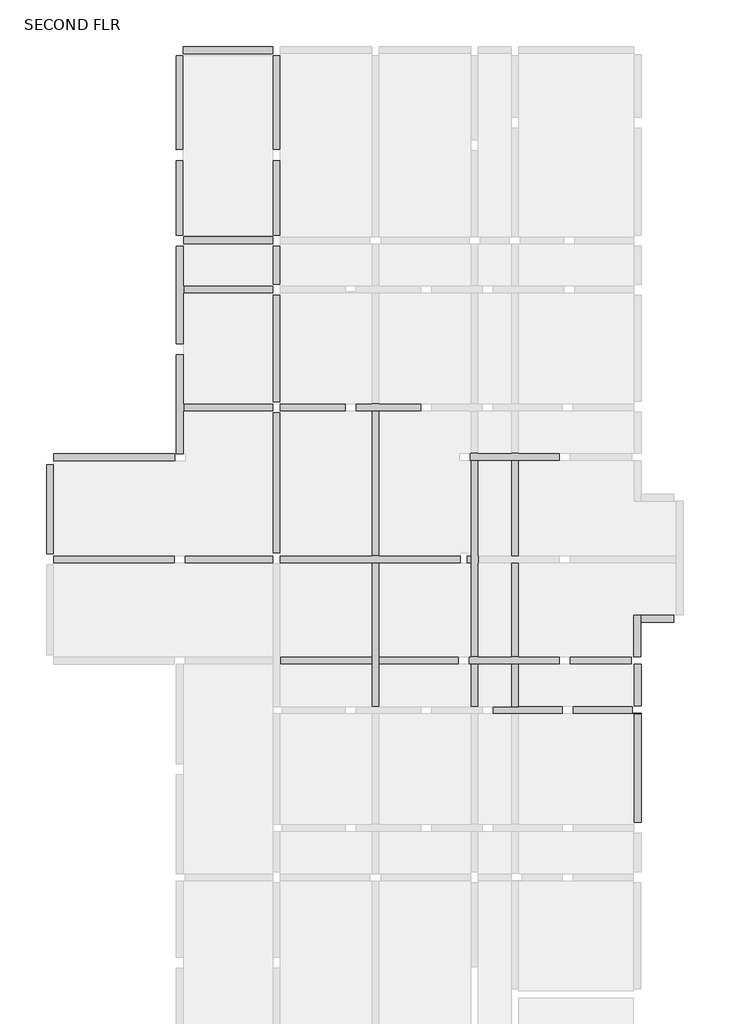
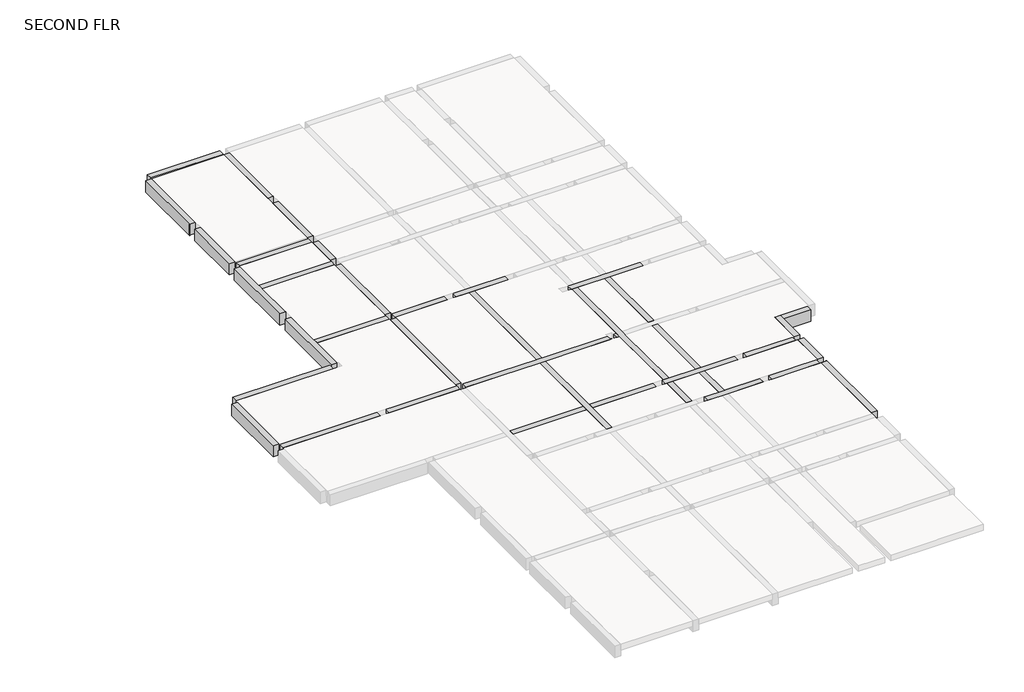
# One storey, part 3 of 4: 39 beams.
"""IFC4 building model written with IfcOpenShell, lengths in millimetres."""

from ifc_helpers import new_model, si_unit, frame, origin, place, context, project, spatial, polyline, outline, extrude, faceted_brep, element, save

model = new_model("IFC4")

# Units and contexts
model_context = context("Model", 3, world=origin())
ifc_project = project(units=[si_unit("LENGTHUNIT", "METRE", prefix="MILLI")], contexts=[model_context])

# Site, building, storey
site = spatial("IfcSite", under=ifc_project)
building = spatial("IfcBuilding", under=site)
storey = spatial("IfcBuildingStorey", under=building, Name="SECOND FLR", Elevation=6048.0)

# Beams
placement = place(None, origin())
element("IfcBeam", 1, ObjectType="M_Concrete-Rectangular Beam : 300 x 600mm", at=placement, inside=storey, context=model_context, shape_type="SweptSolid", body=[
    extrude(outline(polyline([(-1971.7865686, 21837.8349362), (-1971.7865686, 21537.8349362), (-5591.7865686, 21537.8349362), (-5591.7865686, 21837.8349362), (-1971.7865686, 21837.8349362)])), frame((0.0, 0.0, 5448.0), z_axis=(0.0, 0.0, 1.0), x_axis=(1.0, 0.0, 0.0)), (0.0, 0.0, 1.0), 600.0),
])
element("IfcBeam", 2, ObjectType="M_Concrete-Rectangular Beam : 300 x 600mm", at=placement, inside=storey, context=model_context, shape_type="Brep", body=[
    faceted_brep([(-5891.7865686, 21462.8349362, 6048.0), (-5891.7865686, 17662.8349362, 6048.0), (-5888.8105653, 17662.8349362, 6048.0), (-5888.8105653, 17674.7148651, 6048.0), (-5591.7865686, 17674.7148651, 6048.0), (-5591.7865686, 21462.8349362, 6048.0), (-5891.7865686, 21462.8349362, 5448.0), (-5891.7865686, 17662.8349362, 5448.0), (-5591.7865686, 21462.8349362, 5448.0), (-5591.7865686, 17674.7148651, 5448.0), (-5888.8105653, 17674.7148651, 5448.0), (-5888.8105653, 17662.8349362, 5448.0), (-5591.7865686, 17674.7148651, 5748.0), (-5591.7865686, 21462.8349362, 5748.0)], [[[0, 1, 2, 3, 4, 5]], [[1, 0, 6, 7]], [[7, 6, 8, 9, 10, 11]], [[5, 4, 12, 9, 8, 13]], [[8, 6, 0, 5, 13]], [[1, 7, 11, 2]], [[10, 3, 2, 11]], [[3, 10, 9, 12, 4]]]),
])
element("IfcBeam", 3, ObjectType="M_Concrete-Rectangular Beam : 300 x 600mm", at=placement, inside=storey, context=model_context, shape_type="SweptSolid", body=[
    extrude(outline(polyline([(6048.0, -5888.8105653), (5448.0, -5888.8105653), (5448.0, -5588.8105653), (5748.0, -5588.8105653), (5748.0, -5591.7865686), (6048.0, -5591.7865686), (6048.0, -5888.8105653)])), frame((0.0, 14212.5179708, 0.0), z_axis=(0.0, 1.0, 0.0), x_axis=(0.0, 0.0, 1.0)), (0.0, 0.0, 1.0), 3012.1968944),
])
element("IfcBeam", 4, ObjectType="M_Concrete-Rectangular Beam : 300 x 600mm", at=placement, inside=storey, context=model_context, shape_type="Brep", body=[
    faceted_brep([(-5888.8105653, 13762.5179708, 6048.0), (-5888.8105653, 9817.5252033, 6048.0), (-5588.8105653, 9817.5252033, 6048.0), (-5588.8105653, 11857.4075451, 6048.0), (-5588.8105653, 12157.4075451, 6048.0), (-5588.8105653, 13762.5179708, 6048.0), (-5888.8105653, 13762.5179708, 5448.0), (-5888.8105653, 9817.5252033, 5448.0), (-5588.8105653, 13762.5179708, 5448.0), (-5588.8105653, 12157.4075451, 5448.0), (-5588.8105653, 11857.4075451, 5448.0), (-5588.8105653, 9817.5252033, 5448.0), (-5588.8105653, 13762.5179708, 5748.0), (-5588.8105653, 9817.5252033, 5748.0)], [[[0, 1, 2, 3, 4, 5]], [[1, 0, 6, 7]], [[7, 6, 8, 9, 10, 11]], [[11, 10, 9, 8, 12, 5, 4, 3, 2, 13]], [[8, 6, 0, 5, 12]], [[2, 1, 7, 11, 13]]]),
])
element("IfcBeam", 5, ObjectType="M_Concrete-Rectangular Beam : 300 x 600mm", at=placement, inside=storey, context=model_context, shape_type="Brep", body=[
    faceted_brep([(-5888.8105653, 9367.5252033, 6048.0), (-5888.8105653, 5367.5252033, 6048.0), (-5588.8105653, 5367.5252033, 6048.0), (-5588.8105653, 7099.7076276, 6048.0), (-5588.8105653, 7399.7076276, 6048.0), (-5588.8105653, 9367.5252033, 6048.0), (-5888.8105653, 9367.5252033, 5448.0), (-5888.8105653, 5367.5252033, 5448.0), (-5588.8105653, 9367.5252033, 5448.0), (-5588.8105653, 7399.7076276, 5448.0), (-5588.8105653, 7099.7076276, 5448.0), (-5588.8105653, 5367.5252033, 5448.0), (-5588.8105653, 9367.5252033, 5748.0), (-5588.8105653, 5367.5252033, 5748.0)], [[[0, 1, 2, 3, 4, 5]], [[1, 0, 6, 7]], [[7, 6, 8, 9, 10, 11]], [[11, 10, 9, 8, 12, 5, 4, 3, 2, 13]], [[8, 6, 0, 5, 12]], [[2, 1, 7, 11, 13]]]),
])
element("IfcBeam", 6, ObjectType="M_Concrete-Rectangular Beam : 300 x 600mm", at=placement, inside=storey, context=model_context, shape_type="Brep", body=[
    faceted_brep([(-5943.8105653, 5067.6057249, 6048.0), (-5943.8105653, 5367.6057249, 6048.0), (-10828.8105653, 5367.6057249, 6048.0), (-10828.8105653, 5067.6057249, 6048.0), (-5943.8105653, 5367.6057249, 5448.0), (-10828.8105653, 5367.6057249, 5448.0), (-5943.8105653, 5067.6057249, 5448.0), (-10828.8105653, 5067.6057249, 5448.0), (-10828.8105653, 5067.6057249, 5748.0), (-5943.8105653, 5067.6057249, 5748.0)], [[[0, 1, 2, 3]], [[1, 4, 5, 2]], [[4, 6, 7, 5]], [[0, 3, 8, 7, 6, 9]], [[6, 4, 1, 0, 9]], [[3, 2, 5, 7, 8]]]),
])
element("IfcBeam", 7, ObjectType="M_Concrete-Rectangular Beam : 300 x 600mm", at=placement, inside=storey, context=model_context, shape_type="SweptSolid", body=[
    extrude(outline(polyline([(-10828.8105653, 1326.1713929), (-11128.8105653, 1326.1713929), (-11128.8105653, 4932.6057249), (-10828.8105653, 4932.6057249), (-10828.8105653, 1326.1713929)])), frame((0.0, 0.0, 5448.0), z_axis=(0.0, 0.0, 1.0), x_axis=(1.0, 0.0, 0.0)), (0.0, 0.0, 1.0), 600.0),
])
element("IfcBeam", 8, ObjectType="M_Concrete-Rectangular Beam : 300 x 600mm", at=placement, inside=storey, context=model_context, shape_type="Brep", body=[
    faceted_brep([(12619.1163908, -5144.3229916, 6048.0), (12919.1163908, -5144.3229916, 6048.0), (12919.1163908, -5144.3229916, 5448.0), (12619.1163908, -5144.3229916, 5448.0), (12619.1163908, -5151.6229916, 6048.0), (12619.1163908, -9532.1078267, 6048.0), (12919.1163908, -9532.1078267, 6048.0), (12919.1163908, -9532.1078267, 5448.0), (12619.1163908, -9532.1078267, 5448.0), (12619.1163908, -5151.6229916, 5448.0), (12619.1163908, -9532.1078267, 5748.0)], [[[0, 1, 2, 3]], [[1, 0, 4, 5, 6]], [[2, 1, 6, 7]], [[3, 2, 7, 8, 9]], [[0, 3, 9, 8, 10, 5, 4]], [[8, 7, 6, 5, 10]]]),
])
element("IfcBeam", 9, ObjectType="M_Concrete-Rectangular Beam : 300 x 600mm", at=placement, inside=storey, context=model_context, shape_type="Brep", body=[
    faceted_brep([(12619.1163908, -4818.9229916, 5448.0), (12919.1163908, -4818.9229916, 5448.0), (12919.1163908, -4818.9229916, 6048.0), (12619.1163908, -4818.9229916, 6048.0), (12619.1163908, -4818.9229916, 5748.0), (12919.1163908, -3139.4535766, 6048.0), (12619.1163908, -3139.4535766, 6048.0), (12919.1163908, -3139.4535766, 5448.0), (12619.1163908, -3139.4535766, 5448.0), (12619.1163908, -3139.4535766, 5748.0)], [[[0, 1, 2, 3, 4]], [[3, 2, 5, 6]], [[2, 1, 7, 5]], [[1, 0, 8, 7]], [[3, 6, 9, 8, 0, 4]], [[6, 5, 7, 8, 9]]]),
])
element("IfcBeam", 10, ObjectType="M_Concrete-Rectangular Beam : 300 x 600mm", at=placement, inside=storey, context=model_context, shape_type="Brep", body=[
    faceted_brep([(12599.1163908, -2839.4535766, 6048.0), (12899.1163908, -2839.4535766, 6048.0), (12899.1163908, -1448.8286071, 6048.0), (12899.1163908, -1148.8286071, 6048.0), (12599.1163908, -1148.8286071, 6048.0), (12899.1163908, -2839.4535766, 5448.0), (12899.1163908, -1448.8286071, 5448.0), (12899.1163908, -1148.8286071, 5448.0), (12899.1163908, -1148.8286071, 5748.0), (12599.1163908, -2839.4535766, 5448.0), (12599.1163908, -1148.8286071, 5448.0), (12599.1163908, -1148.8286071, 5748.0), (12599.1163908, -2839.4535766, 5748.0)], [[[0, 1, 2, 3, 4]], [[1, 5, 6, 7, 8, 3, 2]], [[5, 9, 10, 7, 6]], [[0, 4, 11, 10, 9, 12]], [[9, 5, 1, 0, 12]], [[4, 3, 8, 7, 10, 11]]]),
])
element("IfcBeam", 11, ObjectType="M_Concrete-Rectangular Beam : 300 x 600mm", at=placement, inside=storey, context=model_context, shape_type="Brep", body=[
    faceted_brep([(14244.1163908, -1448.8286071, 6048.0), (14244.1163908, -1148.8286071, 6048.0), (12899.1163908, -1148.8286071, 6048.0), (12899.1163908, -1448.8286071, 6048.0), (14244.1163908, -1148.8286071, 5748.0), (14244.1163908, -1148.8286071, 5448.0), (12899.1163908, -1148.8286071, 5448.0), (12899.1163908, -1148.8286071, 5748.0), (14244.1163908, -1448.8286071, 5448.0), (12899.1163908, -1448.8286071, 5448.0)], [[[0, 1, 2, 3]], [[2, 1, 4, 5, 6, 7]], [[5, 8, 9, 6]], [[8, 0, 3, 9]], [[0, 8, 5, 4, 1]], [[3, 2, 7, 6, 9]]]),
])
element("IfcBeam", 12, ObjectType="M_Concrete-Rectangular Beam : 300 x 600mm", at=placement, inside=storey, context=model_context, shape_type="Brep", body=[
    faceted_brep([(-1671.7865686, 21462.8349362, 6048.0), (-1971.7865686, 21462.8349362, 6048.0), (-1971.7865686, 17674.7148651, 6048.0), (-1671.7865686, 17674.7148651, 6048.0), (-1971.7865686, 21462.8349362, 5748.0), (-1971.7865686, 21462.8349362, 5448.0), (-1971.7865686, 17674.7148651, 5448.0), (-1971.7865686, 17674.7148651, 5748.0), (-1671.7865686, 21462.8349362, 5448.0), (-1671.7865686, 17674.7148651, 5448.0), (-1671.7865686, 17674.7148651, 5748.0), (-1671.7865686, 21462.8349362, 5748.0)], [[[0, 1, 2, 3]], [[2, 1, 4, 5, 6, 7]], [[5, 8, 9, 6]], [[0, 3, 10, 9, 8, 11]], [[1, 0, 11, 8, 5, 4]], [[3, 2, 7, 6, 9, 10]]]),
])
element("IfcBeam", 13, ObjectType="M_Concrete-Rectangular Beam : 300 x 600mm", at=placement, inside=storey, context=model_context, shape_type="Brep", body=[
    faceted_brep([(-1671.7865686, 17224.7148651, 6048.0), (-1971.7865686, 17224.7148651, 6048.0), (-1971.7865686, 14212.5179708, 6048.0), (-1671.7865686, 14212.5179708, 6048.0), (-1971.7865686, 17224.7148651, 5748.0), (-1971.7865686, 17224.7148651, 5448.0), (-1971.7865686, 14212.5179708, 5448.0), (-1971.7865686, 14212.5179708, 5748.0), (-1671.7865686, 17224.7148651, 5448.0), (-1671.7865686, 14212.5179708, 5448.0), (-1671.7865686, 14212.5179708, 5748.0), (-1671.7865686, 17224.7148651, 5748.0)], [[[0, 1, 2, 3]], [[2, 1, 4, 5, 6, 7]], [[5, 8, 9, 6]], [[0, 3, 10, 9, 8, 11]], [[1, 0, 11, 8, 5, 4]], [[3, 2, 7, 6, 9, 10]]]),
])
element("IfcBeam", 14, ObjectType="M_Concrete-Rectangular Beam : 300 x 600mm", at=placement, inside=storey, context=model_context, shape_type="Brep", body=[
    faceted_brep([(-1671.7865686, 13762.5179708, 6048.0), (-1971.7865686, 13762.5179708, 6048.0), (-1971.7865686, 12232.4075451, 6048.0), (-1671.7865686, 12232.4075451, 6048.0), (-1971.7865686, 13762.5179708, 5748.0), (-1971.7865686, 13762.5179708, 5448.0), (-1971.7865686, 12232.4075451, 5448.0), (-1971.7865686, 12232.4075451, 5748.0), (-1671.7865686, 13762.5179708, 5448.0), (-1671.7865686, 12232.4075451, 5448.0), (-1671.7865686, 12232.4075451, 5748.0), (-1671.7865686, 13762.5179708, 5748.0)], [[[0, 1, 2, 3]], [[2, 1, 4, 5, 6, 7]], [[5, 8, 9, 6]], [[0, 3, 10, 9, 8, 11]], [[1, 0, 11, 8, 5, 4]], [[3, 2, 7, 6, 9, 10]]]),
])
element("IfcBeam", 15, ObjectType="M_Concrete-Rectangular Beam : 300 x 600mm", at=placement, inside=storey, context=model_context, shape_type="Brep", body=[
    faceted_brep([(-1671.7865686, 11782.4075451, 6048.0), (-1971.7865686, 11782.4075451, 6048.0), (-1971.7865686, 7474.7076276, 6048.0), (-1671.7865686, 7474.7076276, 6048.0), (-1971.7865686, 11782.4075451, 5748.0), (-1971.7865686, 11782.4075451, 5448.0), (-1971.7865686, 7474.7076276, 5448.0), (-1971.7865686, 7474.7076276, 5748.0), (-1671.7865686, 11782.4075451, 5448.0), (-1671.7865686, 7474.7076276, 5448.0), (-1671.7865686, 7474.7076276, 5748.0), (-1671.7865686, 11782.4075451, 5748.0)], [[[0, 1, 2, 3]], [[2, 1, 4, 5, 6, 7]], [[5, 8, 9, 6]], [[0, 3, 10, 9, 8, 11]], [[1, 0, 11, 8, 5, 4]], [[3, 2, 7, 6, 9, 10]]]),
])
element("IfcBeam", 16, ObjectType="M_Concrete-Rectangular Beam : 300 x 600mm", at=placement, inside=storey, context=model_context, shape_type="Brep", body=[
    faceted_brep([(-1671.7865686, 7024.7076276, 6048.0), (-1971.7865686, 7024.7076276, 6048.0), (-1971.7865686, 1366.1713929, 6048.0), (-1671.7865686, 1366.1713929, 6048.0), (-1971.7865686, 7024.7076276, 5748.0), (-1971.7865686, 7024.7076276, 5448.0), (-1971.7865686, 1366.1713929, 5448.0), (-1971.7865686, 1366.1713929, 5748.0), (-1671.7865686, 7024.7076276, 5448.0), (-1671.7865686, 1366.1713929, 5448.0), (-1671.7865686, 1366.1713929, 5748.0), (-1671.7865686, 7024.7076276, 5748.0)], [[[0, 1, 2, 3]], [[2, 1, 4, 5, 6, 7]], [[5, 8, 9, 6]], [[0, 3, 10, 9, 8, 11]], [[1, 0, 11, 8, 5, 4]], [[3, 2, 7, 6, 9, 10]]]),
])
element("IfcBeam", 17, ObjectType="M_Concrete-Rectangular Beam : 300 x 600mm", at=placement, inside=storey, context=model_context, shape_type="Brep", body=[
    faceted_brep([(-5588.8105653, 14137.5179708, 6048.0), (-5588.8105653, 13837.5179708, 6048.0), (-1971.7865686, 13837.5179708, 6048.0), (-1971.7865686, 14137.5179708, 6048.0), (-5588.8105653, 13837.5179708, 5748.0), (-5588.8105653, 13837.5179708, 5448.0), (-1971.7865686, 13837.5179708, 5448.0), (-1971.7865686, 13837.5179708, 5748.0), (-5588.8105653, 14137.5179708, 5448.0), (-1971.7865686, 14137.5179708, 5448.0)], [[[0, 1, 2, 3]], [[2, 1, 4, 5, 6, 7]], [[5, 8, 9, 6]], [[8, 0, 3, 9]], [[1, 0, 8, 5, 4]], [[9, 3, 2, 7, 6]]]),
])
element("IfcBeam", 18, ObjectType="M_Concrete-Rectangular Beam : 300 x 600mm", at=placement, inside=storey, context=model_context, shape_type="Brep", body=[
    faceted_brep([(-1971.7865686, 11857.4075451, 6048.0), (-1971.7865686, 12157.4075451, 6048.0), (-5588.8105653, 12157.4075451, 6048.0), (-5588.8105653, 11857.4075451, 6048.0), (-5588.8105653, 11857.4075451, 5748.0), (-5588.8105653, 11857.4075451, 5448.0), (-1971.7865686, 11857.4075451, 5448.0), (-1971.7865686, 11857.4075451, 5748.0), (-1971.7865686, 12157.4075451, 5448.0), (-5588.8105653, 12157.4075451, 5448.0), (-1971.7865686, 12157.4075451, 5748.0), (-5588.8105653, 12157.4075451, 5748.0)], [[[0, 1, 2, 3]], [[0, 3, 4, 5, 6, 7]], [[8, 6, 5, 9]], [[2, 1, 10, 8, 9, 11]], [[1, 0, 7, 6, 8, 10]], [[3, 2, 11, 9, 5, 4]]]),
])
element("IfcBeam", 19, ObjectType="M_Concrete-Rectangular Beam : 300 x 600mm", at=placement, inside=storey, context=model_context, shape_type="Brep", body=[
    faceted_brep([(-1971.7865686, 7099.7076276, 6048.0), (-1971.7865686, 7399.7076276, 6048.0), (-5588.8105653, 7399.7076276, 6048.0), (-5588.8105653, 7099.7076276, 6048.0), (-5588.8105653, 7099.7076276, 5748.0), (-5588.8105653, 7099.7076276, 5448.0), (-1971.7865686, 7099.7076276, 5448.0), (-1971.7865686, 7099.7076276, 5748.0), (-1971.7865686, 7399.7076276, 5448.0), (-5588.8105653, 7399.7076276, 5448.0), (-1971.7865686, 7399.7076276, 5748.0), (-5588.8105653, 7399.7076276, 5748.0)], [[[0, 1, 2, 3]], [[0, 3, 4, 5, 6, 7]], [[8, 6, 5, 9]], [[2, 1, 10, 8, 9, 11]], [[1, 0, 7, 6, 8, 10]], [[3, 2, 11, 9, 5, 4]]]),
])
element("IfcBeam", 20, ObjectType="M_Concrete-Rectangular Beam : 300 x 600mm", at=placement, inside=storey, context=model_context, shape_type="Brep", body=[
    faceted_brep([(-1671.7865686, 7399.7076276, 6048.0), (-1671.7865686, 7099.7076276, 6048.0), (949.7296816, 7099.7076276, 6048.0), (949.7296816, 7399.7076276, 6048.0), (-1671.7865686, 7099.7076276, 5748.0), (-1671.7865686, 7099.7076276, 5448.0), (949.7296816, 7099.7076276, 5448.0), (949.7296816, 7099.7076276, 5748.0), (-1671.7865686, 7399.7076276, 5448.0), (949.7296816, 7399.7076276, 5448.0), (949.7296816, 7399.7076276, 5748.0), (-1671.7865686, 7399.7076276, 5748.0)], [[[0, 1, 2, 3]], [[2, 1, 4, 5, 6, 7]], [[5, 8, 9, 6]], [[0, 3, 10, 9, 8, 11]], [[1, 0, 11, 8, 5, 4]], [[3, 2, 7, 6, 9, 10]]]),
])
element("IfcBeam", 21, ObjectType="M_Concrete-Rectangular Beam : 300 x 600mm", at=placement, inside=storey, context=model_context, shape_type="Brep", body=[
    faceted_brep([(1399.7296816, 7399.7076276, 6048.0), (1399.7296816, 7099.7076276, 6048.0), (2024.7296816, 7099.7076276, 6048.0), (2324.7296816, 7099.7076276, 6048.0), (3997.5248054, 7099.7076276, 6048.0), (3997.5248054, 7399.7076276, 6048.0), (2324.7296816, 7399.7076276, 6048.0), (2024.7296816, 7399.7076276, 6048.0), (1399.7296816, 7099.7076276, 5448.0), (2024.7296816, 7099.7076276, 5448.0), (2324.7296816, 7099.7076276, 5448.0), (3997.5248054, 7099.7076276, 5448.0), (3997.5248054, 7099.7076276, 5748.0), (1399.7296816, 7099.7076276, 5748.0), (1399.7296816, 7399.7076276, 5448.0), (2024.7296816, 7399.7076276, 5448.0), (2324.7296816, 7399.7076276, 5448.0), (3997.5248054, 7399.7076276, 5448.0), (1399.7296816, 7399.7076276, 5748.0), (3997.5248054, 7399.7076276, 5748.0)], [[[0, 1, 2, 3, 4, 5, 6, 7]], [[8, 9, 10, 11, 12, 4, 3, 2, 1, 13]], [[8, 14, 15, 16, 17, 11, 10, 9]], [[17, 16, 15, 14, 18, 0, 7, 6, 5, 19]], [[1, 0, 18, 14, 8, 13]], [[5, 4, 12, 11, 17, 19]]]),
])
element("IfcBeam", 22, ObjectType="M_Concrete-Rectangular Beam : 300 x 600mm", at=placement, inside=storey, context=model_context, shape_type="Brep", body=[
    faceted_brep([(6007.5248054, 5387.6057249, 6048.0), (6007.5248054, 5087.6057249, 6048.0), (6032.5248054, 5087.6057249, 6048.0), (6332.5248054, 5087.6057249, 6048.0), (7656.8679014, 5087.6057249, 6048.0), (7956.8679014, 5087.6057249, 6048.0), (9601.8679014, 5087.6057249, 6048.0), (9601.8679014, 5387.6057249, 6048.0), (7956.8679014, 5387.6057249, 6048.0), (7656.8679014, 5387.6057249, 6048.0), (6332.5248054, 5387.6057249, 6048.0), (6032.5248054, 5387.6057249, 6048.0), (6007.5248054, 5087.6057249, 5448.0), (6032.5248054, 5087.6057249, 5448.0), (6332.5248054, 5087.6057249, 5448.0), (7656.8679014, 5087.6057249, 5448.0), (7956.8679014, 5087.6057249, 5448.0), (9601.8679014, 5087.6057249, 5448.0), (9601.8679014, 5087.6057249, 5748.0), (6007.5248054, 5087.6057249, 5748.0), (6007.5248054, 5387.6057249, 5448.0), (6032.5248054, 5387.6057249, 5448.0), (6332.5248054, 5387.6057249, 5448.0), (7656.8679014, 5387.6057249, 5448.0), (7956.8679014, 5387.6057249, 5448.0), (9601.8679014, 5387.6057249, 5448.0), (6007.5248054, 5387.6057249, 5748.0), (9601.8679014, 5387.6057249, 5748.0)], [[[0, 1, 2, 3, 4, 5, 6, 7, 8, 9, 10, 11]], [[12, 13, 14, 15, 16, 17, 18, 6, 5, 4, 3, 2, 1, 19]], [[12, 20, 21, 22, 23, 24, 25, 17, 16, 15, 14, 13]], [[25, 24, 23, 22, 21, 20, 26, 0, 11, 10, 9, 8, 7, 27]], [[1, 0, 26, 20, 12, 19]], [[7, 6, 18, 17, 25, 27]]]),
])
element("IfcBeam", 23, ObjectType="M_Concrete-Rectangular Beam : 300 x 600mm", at=placement, inside=storey, context=model_context, shape_type="Brep", body=[
    faceted_brep([(-10828.8105653, 1251.1713929, 6048.0), (-10828.8105653, 951.1713929, 6048.0), (-5963.8105653, 951.1713929, 6048.0), (-5963.8105653, 1251.1713929, 6048.0), (-10828.8105653, 951.1713929, 5748.0), (-10828.8105653, 951.1713929, 5448.0), (-5963.8105653, 951.1713929, 5448.0), (-5963.8105653, 951.1713929, 5748.0), (-10828.8105653, 1251.1713929, 5448.0), (-5963.8105653, 1251.1713929, 5448.0), (-5963.8105653, 1251.1713929, 5748.0), (-10828.8105653, 1251.1713929, 5748.0)], [[[0, 1, 2, 3]], [[2, 1, 4, 5, 6, 7]], [[5, 8, 9, 6]], [[0, 3, 10, 9, 8, 11]], [[1, 0, 11, 8, 5, 4]], [[3, 2, 7, 6, 9, 10]]]),
])
element("IfcBeam", 24, ObjectType="M_Concrete-Rectangular Beam : 300 x 600mm", at=placement, inside=storey, context=model_context, shape_type="Brep", body=[
    faceted_brep([(-5513.8105653, 1251.1713929, 6048.0), (-5513.8105653, 951.1713929, 6048.0), (-1971.7865686, 951.1713929, 6048.0), (-1971.7865686, 1251.1713929, 6048.0), (-5513.8105653, 951.1713929, 5748.0), (-5513.8105653, 951.1713929, 5448.0), (-1971.7865686, 951.1713929, 5448.0), (-1971.7865686, 951.1713929, 5748.0), (-5513.8105653, 1251.1713929, 5448.0), (-1971.7865686, 1251.1713929, 5448.0), (-1971.7865686, 1251.1713929, 5748.0), (-5513.8105653, 1251.1713929, 5748.0)], [[[0, 1, 2, 3]], [[2, 1, 4, 5, 6, 7]], [[5, 8, 9, 6]], [[0, 3, 10, 9, 8, 11]], [[1, 0, 11, 8, 5, 4]], [[3, 2, 7, 6, 9, 10]]]),
])
element("IfcBeam", 25, ObjectType="M_Concrete-Rectangular Beam : 300 x 600mm", at=placement, inside=storey, context=model_context, shape_type="Brep", body=[
    faceted_brep([(9601.8679014, -3139.4535766, 6048.0), (9601.8679014, -2839.4535766, 6048.0), (7956.8679014, -2839.4535766, 6048.0), (7656.8679014, -2839.4535766, 6048.0), (6332.5248054, -2839.4535766, 6048.0), (6032.5248054, -2839.4535766, 6048.0), (5967.5248054, -2839.4535766, 6048.0), (5967.5248054, -3139.4535766, 6048.0), (6032.5248054, -3139.4535766, 6048.0), (6332.5248054, -3139.4535766, 6048.0), (7656.8679014, -3139.4535766, 6048.0), (7956.8679014, -3139.4535766, 6048.0), (5967.5248054, -3139.4535766, 5448.0), (6032.5248054, -3139.4535766, 5448.0), (6332.5248054, -3139.4535766, 5448.0), (7656.8679014, -3139.4535766, 5448.0), (7956.8679014, -3139.4535766, 5448.0), (9601.8679014, -3139.4535766, 5448.0), (9601.8679014, -3139.4535766, 5748.0), (5967.5248054, -3139.4535766, 5748.0), (9601.8679014, -2839.4535766, 5448.0), (5967.5248054, -2839.4535766, 5448.0), (6032.5248054, -2839.4535766, 5448.0), (6332.5248054, -2839.4535766, 5448.0), (7656.8679014, -2839.4535766, 5448.0), (7956.8679014, -2839.4535766, 5448.0), (5967.5248054, -2839.4535766, 5748.0), (9601.8679014, -2839.4535766, 5748.0)], [[[0, 1, 2, 3, 4, 5, 6, 7, 8, 9, 10, 11]], [[12, 13, 14, 15, 16, 17, 18, 0, 11, 10, 9, 8, 7, 19]], [[20, 17, 16, 15, 14, 13, 12, 21, 22, 23, 24, 25]], [[20, 25, 24, 23, 22, 21, 26, 6, 5, 4, 3, 2, 1, 27]], [[1, 0, 18, 17, 20, 27]], [[7, 6, 26, 21, 12, 19]]]),
])
element("IfcBeam", 26, ObjectType="M_Concrete-Rectangular Beam : 300 x 600mm", at=placement, inside=storey, context=model_context, shape_type="Brep", body=[
    faceted_brep([(12524.1163908, -3139.4535766, 6048.0), (12524.1163908, -2839.4535766, 6048.0), (10051.8679014, -2839.4535766, 6048.0), (10051.8679014, -3139.4535766, 6048.0), (10051.8679014, -3139.4535766, 5748.0), (10051.8679014, -3139.4535766, 5448.0), (12524.1163908, -3139.4535766, 5448.0), (12524.1163908, -3139.4535766, 5748.0), (12524.1163908, -2839.4535766, 5448.0), (10051.8679014, -2839.4535766, 5448.0), (12524.1163908, -2839.4535766, 5748.0), (10051.8679014, -2839.4535766, 5748.0)], [[[0, 1, 2, 3]], [[0, 3, 4, 5, 6, 7]], [[8, 6, 5, 9]], [[2, 1, 10, 8, 9, 11]], [[1, 0, 7, 6, 8, 10]], [[3, 2, 11, 9, 5, 4]]]),
])
element("IfcBeam", 27, ObjectType="M_Concrete-Rectangular Beam : 300 x 600mm", at=placement, inside=storey, context=model_context, shape_type="Brep", body=[
    faceted_brep([(6931.8679014, -4851.6229916, 6048.0), (6931.8679014, -5151.6229916, 6048.0), (7656.8679014, -5151.6229916, 6048.0), (7956.8679014, -5151.6229916, 6048.0), (9721.8679014, -5151.6229916, 6048.0), (9721.8679014, -4851.6229916, 6048.0), (7956.8679014, -4851.6229916, 6048.0), (7656.8679014, -4851.6229916, 6048.0), (6931.8679014, -5151.6229916, 5448.0), (7656.8679014, -5151.6229916, 5448.0), (7956.8679014, -5151.6229916, 5448.0), (9721.8679014, -5151.6229916, 5448.0), (9721.8679014, -5151.6229916, 5748.0), (6931.8679014, -5151.6229916, 5748.0), (6931.8679014, -4851.6229916, 5448.0), (7656.8679014, -4851.6229916, 5448.0), (7956.8679014, -4851.6229916, 5448.0), (9721.8679014, -4851.6229916, 5448.0)], [[[0, 1, 2, 3, 4, 5, 6, 7]], [[8, 9, 10, 11, 12, 4, 3, 2, 1, 13]], [[8, 14, 15, 16, 17, 11, 10, 9]], [[14, 0, 7, 6, 5, 17, 16, 15]], [[1, 0, 14, 8, 13]], [[5, 4, 12, 11, 17]]]),
])
element("IfcBeam", 28, ObjectType="M_Concrete-Rectangular Beam : 300 x 600mm", at=placement, inside=storey, context=model_context, shape_type="Brep", body=[
    faceted_brep([(6032.5248054, 951.1713929, 6048.0), (6032.5248054, 1251.1713929, 6048.0), (5892.5248054, 1251.1713929, 6048.0), (5892.5248054, 951.1713929, 6048.0), (5892.5248054, 951.1713929, 5748.0), (5892.5248054, 951.1713929, 5448.0), (6032.5248054, 951.1713929, 5448.0), (6032.5248054, 951.1713929, 5748.0), (6032.5248054, 1251.1713929, 5448.0), (5892.5248054, 1251.1713929, 5448.0), (6032.5248054, 1251.1713929, 5748.0), (5892.5248054, 1251.1713929, 5748.0)], [[[0, 1, 2, 3]], [[0, 3, 4, 5, 6, 7]], [[8, 6, 5, 9]], [[2, 1, 10, 8, 9, 11]], [[1, 0, 7, 6, 8, 10]], [[3, 2, 11, 9, 5, 4]]]),
    faceted_brep([(-1671.7865686, 951.1713929, 6048.0), (-1671.7865686, 1251.1713929, 6048.0), (-1671.7865686, 1251.1713929, 5748.0), (-1671.7865686, 1251.1713929, 5448.0), (-1671.7865686, 951.1713929, 5448.0), (-1671.7865686, 951.1713929, 5748.0), (5592.5248054, 1251.1713929, 6048.0), (5592.5248054, 951.1713929, 6048.0), (5592.5248054, 951.1713929, 5748.0), (5592.5248054, 951.1713929, 5448.0), (5592.5248054, 1251.1713929, 5448.0), (5592.5248054, 1251.1713929, 5748.0), (2024.7296816, 951.1713929, 6048.0), (2324.7296816, 951.1713929, 6048.0), (2324.7296816, 1251.1713929, 6048.0), (2024.7296816, 1251.1713929, 6048.0), (2024.7296816, 951.1713929, 5448.0), (2324.7296816, 951.1713929, 5448.0), (2024.7296816, 1251.1713929, 5448.0), (2324.7296816, 1251.1713929, 5448.0)], [[[0, 1, 2, 3, 4, 5]], [[6, 7, 8, 9, 10, 11]], [[1, 0, 12, 13, 7, 6, 14, 15]], [[4, 16, 17, 9, 8, 7, 13, 12, 0, 5]], [[4, 3, 18, 19, 10, 9, 17, 16]], [[10, 19, 18, 3, 2, 1, 15, 14, 6, 11]]]),
])
element("IfcBeam", 29, ObjectType="M_Concrete-Rectangular Beam : 300 x 600mm", at=placement, inside=storey, context=model_context, shape_type="Brep", body=[
    faceted_brep([(-1671.7865686, -2839.4535766, 6048.0), (-1671.7865686, -3139.4535766, 6048.0), (2024.7296816, -3139.4535766, 6048.0), (2024.7296816, -2839.4535766, 6048.0), (-1671.7865686, -3139.4535766, 5748.0), (-1671.7865686, -3139.4535766, 5448.0), (2024.7296816, -3139.4535766, 5448.0), (2024.7296816, -3139.4535766, 5748.0), (-1671.7865686, -2839.4535766, 5448.0), (2024.7296816, -2839.4535766, 5448.0), (2024.7296816, -2839.4535766, 5748.0), (-1671.7865686, -2839.4535766, 5748.0)], [[[0, 1, 2, 3]], [[2, 1, 4, 5, 6, 7]], [[5, 8, 9, 6]], [[0, 3, 10, 9, 8, 11]], [[1, 0, 11, 8, 5, 4]], [[3, 2, 7, 6, 9, 10]]]),
])
element("IfcBeam", 30, ObjectType="M_Concrete-Rectangular Beam : 300 x 600mm", at=placement, inside=storey, context=model_context, shape_type="Brep", body=[
    faceted_brep([(2324.7296816, 7099.7076276, 6048.0), (2024.7296816, 7099.7076276, 6048.0), (2024.7296816, 1251.1713929, 6048.0), (2324.7296816, 1251.1713929, 6048.0), (2024.7296816, 7099.7076276, 5748.0), (2024.7296816, 7099.7076276, 5448.0), (2024.7296816, 1251.1713929, 5448.0), (2024.7296816, 1251.1713929, 5748.0), (2324.7296816, 7099.7076276, 5448.0), (2324.7296816, 5387.6057249, 5448.0), (2324.7296816, 5087.6057249, 5448.0), (2324.7296816, 1251.1713929, 5448.0), (2324.7296816, 1251.1713929, 5748.0), (2324.7296816, 7099.7076276, 5748.0)], [[[0, 1, 2, 3]], [[2, 1, 4, 5, 6, 7]], [[5, 8, 9, 10, 11, 6]], [[0, 3, 12, 11, 10, 9, 8, 13]], [[1, 0, 13, 8, 5, 4]], [[3, 2, 7, 6, 11, 12]]]),
])
element("IfcBeam", 31, ObjectType="M_Concrete-Rectangular Beam : 300 x 600mm", at=placement, inside=storey, context=model_context, shape_type="Brep", body=[
    faceted_brep([(6332.5248054, 5087.6057249, 6048.0), (6032.5248054, 5087.6057249, 6048.0), (6032.5248054, 1251.1713929, 6048.0), (6032.5248054, 951.1713929, 6048.0), (6032.5248054, -2839.4535766, 6048.0), (6332.5248054, -2839.4535766, 6048.0), (6332.5248054, 951.1713929, 6048.0), (6332.5248054, 1251.1713929, 6048.0), (6032.5248054, 5087.6057249, 5448.0), (6032.5248054, 1251.1713929, 5448.0), (6032.5248054, 951.1713929, 5448.0), (6032.5248054, -2839.4535766, 5448.0), (6032.5248054, -2839.4535766, 5748.0), (6032.5248054, 5087.6057249, 5748.0), (6332.5248054, 5087.6057249, 5448.0), (6332.5248054, 1251.1713929, 5448.0), (6332.5248054, 951.1713929, 5448.0), (6332.5248054, -2839.4535766, 5448.0), (6332.5248054, 5087.6057249, 5748.0), (6332.5248054, -2839.4535766, 5748.0)], [[[0, 1, 2, 3, 4, 5, 6, 7]], [[8, 9, 10, 11, 12, 4, 3, 2, 1, 13]], [[8, 14, 15, 16, 17, 11, 10, 9]], [[17, 16, 15, 14, 18, 0, 7, 6, 5, 19]], [[1, 0, 18, 14, 8, 13]], [[5, 4, 12, 11, 17, 19]]]),
])
element("IfcBeam", 32, ObjectType="M_Concrete-Rectangular Beam : 300 x 600mm", at=placement, inside=storey, context=model_context, shape_type="Brep", body=[
    faceted_brep([(7956.8679014, 5087.6057249, 6048.0), (7656.8679014, 5087.6057249, 6048.0), (7656.8679014, 1251.1713929, 6048.0), (7956.8679014, 1251.1713929, 6048.0), (7656.8679014, 5087.6057249, 5748.0), (7656.8679014, 5087.6057249, 5448.0), (7656.8679014, 1251.1713929, 5448.0), (7656.8679014, 1251.1713929, 5748.0), (7956.8679014, 5087.6057249, 5448.0), (7956.8679014, 1251.1713929, 5448.0), (7956.8679014, 1251.1713929, 5748.0), (7956.8679014, 5087.6057249, 5748.0)], [[[0, 1, 2, 3]], [[2, 1, 4, 5, 6, 7]], [[5, 8, 9, 6]], [[0, 3, 10, 9, 8, 11]], [[1, 0, 11, 8, 5, 4]], [[3, 2, 7, 6, 9, 10]]]),
])
element("IfcBeam", 33, ObjectType="M_Concrete-Rectangular Beam : 300 x 600mm", at=placement, inside=storey, context=model_context, shape_type="Brep", body=[
    faceted_brep([(6332.5248054, -3139.4535766, 6048.0), (6032.5248054, -3139.4535766, 6048.0), (6032.5248054, -4851.6229916, 6048.0), (6332.5248054, -4851.6229916, 6048.0), (6032.5248054, -3139.4535766, 5748.0), (6032.5248054, -3139.4535766, 5448.0), (6032.5248054, -4851.6229916, 5448.0), (6032.5248054, -4851.6229916, 5748.0), (6332.5248054, -3139.4535766, 5448.0), (6332.5248054, -4851.6229916, 5448.0), (6332.5248054, -3139.4535766, 5748.0), (6332.5248054, -4851.6229916, 5748.0)], [[[0, 1, 2, 3]], [[2, 1, 4, 5, 6, 7]], [[5, 8, 9, 6]], [[8, 10, 0, 3, 11, 9]], [[1, 0, 10, 8, 5, 4]], [[3, 2, 7, 6, 9, 11]]]),
])
element("IfcBeam", 34, ObjectType="M_Concrete-Rectangular Beam : 300 x 600mm", at=placement, inside=storey, context=model_context, shape_type="Brep", body=[
    faceted_brep([(7956.8679014, -3139.4535766, 6048.0), (7656.8679014, -3139.4535766, 6048.0), (7656.8679014, -4851.6229916, 6048.0), (7956.8679014, -4851.6229916, 6048.0), (7956.8679014, -4831.6229916, 6048.0), (7656.8679014, -3139.4535766, 5748.0), (7656.8679014, -3139.4535766, 5448.0), (7656.8679014, -4851.6229916, 5448.0), (7656.8679014, -4851.6229916, 5748.0), (7956.8679014, -3139.4535766, 5448.0), (7956.8679014, -4851.6229916, 5448.0), (7956.8679014, -3139.4535766, 5748.0)], [[[0, 1, 2, 3, 4]], [[1, 5, 6, 7, 8, 2]], [[6, 9, 10, 7]], [[10, 9, 11, 0, 4, 3]], [[1, 0, 11, 9, 6, 5]], [[3, 2, 8, 7, 10]]]),
])
element("IfcBeam", 35, ObjectType="M_Concrete-Rectangular Beam : 300 x 600mm", at=placement, inside=storey, context=model_context, shape_type="Brep", body=[
    faceted_brep([(2024.7296816, -4851.6229916, 6048.0), (2324.7296816, -4851.6229916, 6048.0), (2324.7296816, -3139.4535766, 6048.0), (2324.7296816, -2839.4535766, 6048.0), (2324.7296816, 951.1713929, 6048.0), (2024.7296816, 951.1713929, 6048.0), (2024.7296816, -2839.4535766, 6048.0), (2024.7296816, -3139.4535766, 6048.0), (2024.7296816, 951.1713929, 5448.0), (2024.7296816, -2839.4535766, 5448.0), (2024.7296816, -3139.4535766, 5448.0), (2024.7296816, -4851.6229916, 5448.0), (2024.7296816, -4851.6229916, 5748.0), (2024.7296816, 951.1713929, 5748.0), (2324.7296816, -4851.6229916, 5448.0), (2324.7296816, 951.1713929, 5448.0), (2324.7296816, -2839.4535766, 5448.0), (2324.7296816, -3139.4535766, 5448.0), (2324.7296816, 951.1713929, 5748.0), (2324.7296816, -4851.6229916, 5748.0)], [[[0, 1, 2, 3, 4, 5, 6, 7]], [[8, 9, 10, 11, 12, 0, 7, 6, 5, 13]], [[14, 11, 10, 9, 8, 15, 16, 17]], [[14, 17, 16, 15, 18, 4, 3, 2, 1, 19]], [[1, 0, 12, 11, 14, 19]], [[5, 4, 18, 15, 8, 13]]]),
])
element("IfcBeam", 36, ObjectType="M_Concrete-Rectangular Beam : 300 x 600mm", at=placement, inside=storey, context=model_context, shape_type="Brep", body=[
    faceted_brep([(5517.5248054, -3139.4535766, 6048.0), (5517.5248054, -2839.4535766, 6048.0), (2324.7296816, -2839.4535766, 6048.0), (2324.7296816, -3139.4535766, 6048.0), (2324.7296816, -3139.4535766, 5748.0), (2324.7296816, -3139.4535766, 5448.0), (5517.5248054, -3139.4535766, 5448.0), (5517.5248054, -3139.4535766, 5748.0), (5517.5248054, -2839.4535766, 5448.0), (2324.7296816, -2839.4535766, 5448.0), (5517.5248054, -2839.4535766, 5748.0), (2324.7296816, -2839.4535766, 5748.0)], [[[0, 1, 2, 3]], [[0, 3, 4, 5, 6, 7]], [[8, 6, 5, 9]], [[2, 1, 10, 8, 9, 11]], [[1, 0, 7, 6, 8, 10]], [[3, 2, 11, 9, 5, 4]]]),
])
element("IfcBeam", 37, ObjectType="M_Concrete-Rectangular Beam : 300 x 600mm", at=placement, inside=storey, context=model_context, shape_type="Brep", body=[
    faceted_brep([(7656.8679014, -2839.4535766, 6048.0), (7956.8679014, -2839.4535766, 6048.0), (7956.8679014, 951.1713929, 6048.0), (7656.8679014, 951.1713929, 6048.0), (7656.8679014, 951.1713929, 5748.0), (7656.8679014, 951.1713929, 5448.0), (7656.8679014, -2839.4535766, 5448.0), (7656.8679014, -2839.4535766, 5748.0), (7956.8679014, -2839.4535766, 5448.0), (7956.8679014, 951.1713929, 5448.0), (7956.8679014, -2839.4535766, 5748.0), (7956.8679014, 951.1713929, 5748.0)], [[[0, 1, 2, 3]], [[0, 3, 4, 5, 6, 7]], [[8, 6, 5, 9]], [[2, 1, 10, 8, 9, 11]], [[1, 0, 7, 6, 8, 10]], [[3, 2, 11, 9, 5, 4]]]),
])
element("IfcBeam", 38, ObjectType="M_Concrete-Rectangular Beam : 300 x 600mm", at=placement, inside=storey, context=model_context, shape_type="SweptSolid", body=[
    extrude(outline(polyline([(5557.5248054, 5387.6057249), (5557.5248054, 5087.6057249), (2324.7296816, 5087.6057249), (2324.7296816, 5387.6057249), (5557.5248054, 5387.6057249)])), frame((0.0, 0.0, 5448.0), z_axis=(0.0, 0.0, 1.0), x_axis=(1.0, 0.0, 0.0)), (0.0, 0.0, 1.0), 300.0),
])
element("IfcBeam", 39, ObjectType="M_Concrete-Rectangular Beam : 300 x 600mm", at=placement, inside=storey, context=model_context, shape_type="Brep", body=[
    faceted_brep([(10171.8679014, -4851.6229916, 6048.0), (10171.8679014, -5151.6229916, 6048.0), (12619.1163908, -5151.6229916, 6048.0), (12619.1163908, -5144.3229916, 6048.0), (12919.1163908, -5144.3229916, 6048.0), (12919.1163908, -5131.6229916, 6048.0), (12564.1163908, -5131.6229916, 6048.0), (12564.1163908, -4851.6229916, 6048.0), (10171.8679014, -5151.6229916, 5748.0), (10171.8679014, -5151.6229916, 5448.0), (12619.1163908, -5151.6229916, 5448.0), (12619.1163908, -5151.6229916, 5748.0), (10171.8679014, -4851.6229916, 5448.0), (12564.1163908, -4851.6229916, 5448.0), (12564.1163908, -5131.6229916, 5448.0), (12919.1163908, -5131.6229916, 5448.0), (12919.1163908, -5144.3229916, 5448.0), (12619.1163908, -5144.3229916, 5448.0)], [[[0, 1, 2, 3, 4, 5, 6, 7]], [[2, 1, 8, 9, 10, 11]], [[9, 12, 13, 14, 15, 16, 17, 10]], [[12, 0, 7, 13]], [[4, 16, 15, 5]], [[1, 0, 12, 9, 8]], [[3, 17, 16, 4]], [[17, 3, 2, 11, 10]], [[14, 6, 5, 15]], [[6, 14, 13, 7]]]),
])

save(model, "model.ifc")

# Revit data of these elements
# Type "M_Concrete-Rectangular Beam : 300 x 600mm"
#   Length [instance default] = 1524 mm
#   b = 300 mm
#   h = 600 mm
#   Structural Material [instance default] = Concrete, Cast-in-Place gray
#   Assembly Code = ""
# Elements 1, 2, 3, 4, 5, 6, 7, 8, 9, 10, 11, 12, 13, 14, 15, 16, 17, 18, 19, 20, 21, 22, 23, 24, 25, 26, 27, 38, 39 (IfcBeam, "M_Concrete-Rectangular Beam : 300 x 600mm")
#   Structural Material = Concrete, Cast-in-Place gray
#   Phase Created = New Construction
#   Materials on its faces: "Concrete, Cast-in-Place gray"
# Elements 28, 29, 30, 31, 32, 33, 34, 35, 36, 37 (IfcBeam, "M_Concrete-Rectangular Beam : 300 x 600mm")
#   Phase Created = New Construction
#   Materials on its faces: "Concrete, Cast-in-Place gray"
# Materials
#   "Concrete, Cast-in-Place gray": class "Concrete", colour RGB 192 192 192, transparency 0, Description = "Cast-in-place concrete", Cost = 0
